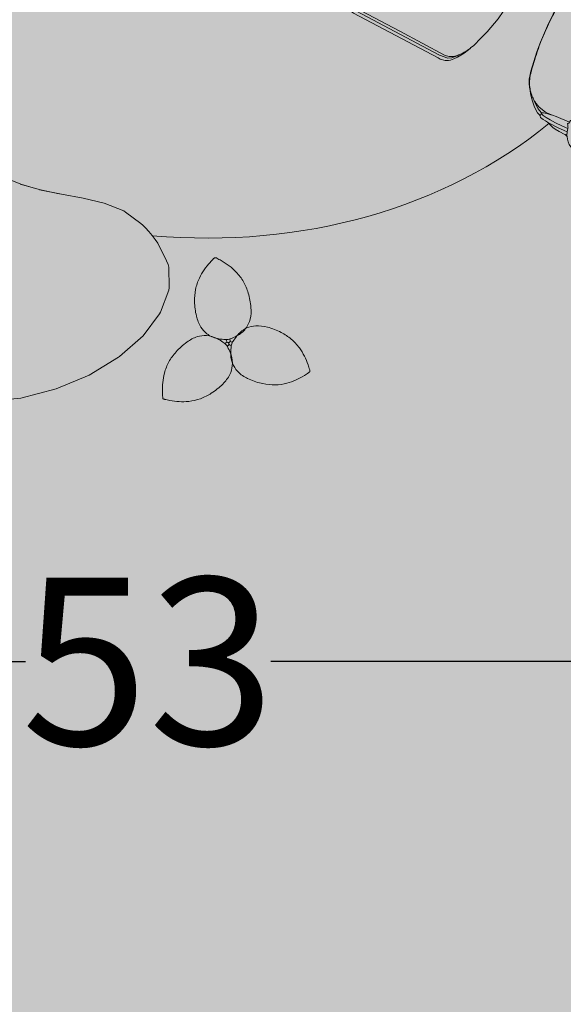
# Model space of a CAD drawing. Units: inches. Extents: x -466983 to 1020, y 324 to 318697.
# Tile 12 of 97: x 775 to 794, y 417 to 452. Entities that reach past the tile are written whole.
import ezdxf

# ---------------------------------------------------------------- set-up
doc = ezdxf.new("R2010")
doc.units = ezdxf.units.IN
doc.header["$MEASUREMENT"] = 0
for name, color, linetype, lineweight in [('A-ANNO-DIMS', 2, 'Continuous', 18), ('A-FLOR-PATT', 252, 'Continuous', 13), ('A-FURN', 8, 'Continuous', 18)]:
    doc.layers.add(name, color=color, linetype=linetype, lineweight=lineweight)
doc.layers.add('K-Hatch', color=7, linetype='Continuous')
doc.styles.get("Standard").update_dxf_attribs({"font": 'arial.ttf'})
doc.dimstyles.get("Standard").update_dxf_attribs({"dimtxt": 6, "dimasz": 4, "dimexe": 3, "dimexo": 3, "dimgap": 0.09, "dimtad": 0, "dimtih": 1, "dimtoh": 1, "dimdec": 1, "dimzin": 0, "dimdsep": 46, "dimlunit": 3, "dimtxsty": 'Standard', "dimcen": 0.09, "dimadec": 0, "dimazin": 0, "dimtfac": 1, "dimtdec": 1, "dimtofl": 0, "dimtmove": 0, "dimatfit": 3, "dimfxl": 1, "dimtolj": 1, "dimtzin": 0, "dimarcsym": 0})

# ---------------------------------------------------------------- blocks, each defined once
blk = doc.blocks.new('CBV_06')
at = {"layer": 'K-Hatch'}
h = blk.add_hatch(color=256, dxfattribs=at)
h.dxf.hatch_style = 1
h.paths.add_polyline_path([(1007.6, -162.8), (976.4, -65), (974.5, -60.9), (923.4, 38), (854.3, 132.5), (771.1, 217.3), (677.3, 287), (580.7, 342.5), (489.2, 384.4), (414.7, 413.4), (369.4, 429.9), (337.4, 440.2), (302.9, 450.6), (264.8, 460.4), (221.9, 468.5), (217.5, 469.1), (173.4, 474.9), (131.2, 477.6), (84.4, 478.5), (-21.2, 478.6), (-84.4, 478.5), (-131.2, 477.6), (-173.4, 474.9), (-217.5, 469.1), (-221.9, 468.5), (-264.8, 460.4), (-302.9, 450.6), (-337.4, 440.2), (-369.4, 429.9), (-414.7, 413.4), (-489.2, 384.4), (-580.7, 342.5), (-677.3, 287), (-771.1, 217.3), (-854.3, 132.5), (-923.4, 38), (-974.5, -60.9), (-976.4, -65), (-1007.6, -162.8), (-1016.4, -252), (-1016.2, -257.5), (-1002.7, -333.7), (-999.3, -339.8), (-963.8, -397.3), (-956.9, -403.9), (-946.2, -410.9), (-945.1, -411.6), (-892.7, -445.8), (-879.3, -451.9), (-863.7, -457.7), (-847.5, -463.3), (-832.6, -467.9), (-820.8, -470.9), (-811.5, -472.7), (-749.7, -478.5), (-742.9, -478.6), (-675.1, -467.1), (-608, -445.9), (-540.7, -420.5), (-533.5, -417.9), (-475.1, -397.7), (-450.5, -390.8), (-411.1, -379.9), (-386, -375.8), (-353.2, -370.6), (-333.2, -368.9), (-297.7, -366.2), (-239.9, -363.6), (-171.9, -362.2), (-95.5, -361.3), (-76.2, -361.4), (-13.7, -361.6), (-21.2, -361.9), (13.7, -361.6), (76.2, -361.4), (95.5, -361.3), (171.9, -362.2), (239.9, -363.6), (297.7, -366.2), (333.2, -368.9), (353.2, -370.6), (386, -375.8), (411.1, -379.9), (450.4, -390.7), (475.1, -397.7), (533.4, -417.9), (540.7, -420.5), (608, -445.9), (675.1, -467.1), (742.9, -478.6), (749.7, -478.5), (811.5, -472.7), (820.8, -470.9), (832.6, -467.9), (847.5, -463.3), (863.7, -457.7), (879.3, -451.9), (892.7, -445.8), (945.1, -411.6), (946.2, -410.9), (956.9, -403.9), (963.8, -397.3), (999.3, -339.8), (1002.7, -333.7), (1016.2, -257.5), (1016.4, -252)])
h.paths.add_polyline_path([(474.4, 70.2), (440.8, 77.6), (404.4, 87.8), (354.2, 104.4), (296.4, 124), (237, 143.3), (236.1, 143.6), (173.2, 161.3), (104.7, 175.8), (50.1, 183.8), (-6.2, 188), (-21.2, 188.7), (-32.5, 186.3), (-104.7, 175.8), (-173.2, 161.3), (-236.1, 143.6), (-237, 143.3), (-296.4, 124), (-354.2, 104.4), (-404.4, 87.8), (-440.8, 77.6), (-474.4, 70.2), (-510.8, 64.3), (-524, 62.5), (-568.6, 59.8), (-577.9, 60.2), (-570.8, 66.8), (-541.1, 87.8), (-513.8, 104.1), (-490.9, 116.3), (-470.5, 126.5), (-453.3, 134.6), (-440.4, 140.4), (-432.6, 143.7), (-427.3, 145.8), (-423.1, 147.3), (-410.5, 149.9), (-379.3, 154.4), (-338.7, 159.3), (-285, 164.8), (-220.8, 170.8), (-21.2, 189.2), (-6.2, 188), (32.5, 186.3), (50.1, 183.8), (220.8, 170.8), (285, 164.8), (338.8, 159.3), (379.3, 154.4), (410.5, 149.9), (423.1, 147.3), (427.3, 145.8), (432.6, 143.7), (440.4, 140.4), (453.3, 134.6), (470.5, 126.5), (490.9, 116.3), (513.8, 104.1), (541.1, 87.8), (570.8, 66.8), (577.9, 60.2), (568.6, 59.8), (524, 62.5), (510.8, 64.3)], flags=16)
for points in [[(472.3, -396.2), (540.7, -420.5), (608, -445.9), (675.1, -467.1), (742.9, -478.6), (749.7, -478.5), (811.5, -472.7), (820.8, -470.9), (832.6, -467.9), (847.5, -463.3), (863.7, -457.7), (879.3, -451.9), (892.7, -445.8), (946.2, -410.9), (956.9, -403.9), (963.8, -397.3), (999.3, -339.8), (1002.7, -333.7), (1016.2, -257.5), (1016.4, -252), (1007.6, -162.8), (976.4, -65), (974.5, -60.9), (923.4, 38), (854.3, 132.5), (771.1, 217.3), (677.3, 287)], [(350, -369.8), (411.1, -379.9), (450.4, -390.7)], [(408.3, -378.8), (475.1, -397.7), (533.4, -417.9)], [(892.7, -445.8), (902.5, -439.6), (946.2, -410.9), (956.9, -403.9)]]:
    blk.add_lwpolyline(points)
blk = doc.blocks.new('CBV_03')
for p, q in [((-46.9, 6), (-51.1, 6)), ((-68.8, -6.7), (-66.7, -3)), ((-58.4, -12.7), (-56.3, -9)), ((-46.9, -6), (-51.1, -6))]:
    blk.add_line(p, q)
blk.add_lwpolyline([(-68.8, 6.7), (-66.7, 3, 1), (-56.3, 9), (-58.4, 12.7)], format="xyb")
for centre, start, end in [((-61.5, -6), 330, 150), ((-51.1, 0), 90, 270)]:
    blk.add_arc(centre, 6, start, end)
for points in [[(-63.3, 9.1), (-67.2, 6.9), (-79, 3.7), (-102.2, -2.7), (-132.8, -0.8), (-164.6, 15.4), (-190.3, 45.3), (-209.9, 82.7), (-222.6, 123.3), (-223.7, 160.5), (-218.2, 193.8), (-210.3, 219.1), (-203.5, 234.1), (-201, 240.5), (-200, 242.1), (-199, 243), (-198.5, 243.3)], [(-63.3, 9.1), (-59.4, 11.4), (-50.7, 20), (-33.6, 36.9), (-19.9, 64.4), (-18.1, 100), (-31.1, 137.2), (-53.6, 172.9), (-82.5, 204.2), (-114.2, 223.8), (-145.8, 235.6), (-171.6, 241.4), (-188, 243.1), (-194.8, 244.1), (-196.7, 244), (-197.9, 243.6), (-198.5, 243.3)], [(-47.4, 0.2), (-47.5, 4.7), (-44.7, 16.6), (-39.2, 40.1), (-22.9, 66), (6.5, 86.2), (45, 94.5), (87.3, 93.9), (129.1, 85.7), (162.2, 68.9), (188.9, 48.1), (207.3, 29.2), (217.3, 16), (221.7, 10.7), (222.6, 9.1), (222.9, 7.8), (222.9, 7.2)], [(-63.3, -9.1), (-67.2, -6.9), (-79, -3.7), (-102.2, 2.7), (-132.8, 0.8), (-164.6, -15.4), (-190.3, -45.3), (-209.9, -82.7), (-222.6, -123.3), (-223.7, -160.5), (-218.2, -193.8), (-210.3, -219.1), (-203.5, -234.1), (-201, -240.5), (-200, -242.1), (-199, -243), (-198.5, -243.3)], [(-47.4, 0.2), (-47.2, -4.3), (-43.8, -16), (-37.2, -39.2), (-19.5, -64.3), (10.9, -82.9), (49.8, -89.2), (91.9, -86.5), (133.3, -76), (165.5, -57.6), (191, -35.4), (208.4, -15.6), (217.7, -1.9), (221.9, 3.6), (222.7, 5.3), (223, 6.6), (222.9, 7.2)], [(-63.3, -9.1), (-59.4, -11.4), (-50.7, -20), (-33.6, -36.9), (-19.9, -64.4), (-18.1, -100), (-31.1, -137.2), (-53.6, -172.9), (-82.5, -204.2), (-114.2, -223.8), (-145.8, -235.6), (-171.6, -241.4), (-188, -243.1), (-194.8, -244.1), (-196.7, -244), (-197.9, -243.6), (-198.5, -243.3)]]:
    blk.add_open_spline(points, degree=3, knots=[0, 0, 0, 0, 13.60379, 35.946241, 72.563034, 102.159646, 140.689545, 188.549731, 228.306921, 267.465056, 298.746796, 329.437779, 346.337038, 348.270011, 350.10195, 352.007195, 352.007195, 352.007195, 352.007195])
blk = doc.blocks.new('CBV_11')
at = {"layer": 'K-Hatch'}
h = blk.add_hatch(color=256, dxfattribs=at)
h.dxf.hatch_style = 1
h.paths.add_polyline_path([(-178.4, 698.3), (-200.4, 717.9), (-207.1, 720), (-213, 721.7), (-231.8, 722.5), (-254.2, 721.5), (-275, 717.7), (-289.3, 712.5), (-316, 699.4), (-324.9, 694.8), (-295.8, 706.5), (-286.8, 709.3), (-277.1, 712.2), (-265.3, 715), (-258.1, 715.9), (-241.3, 718.1), (-228.8, 718), (-215.5, 715.7), (-208.8, 713.2), (-205.5, 711.6), (-203.9, 710.6), (-202.4, 709.7), (-195.4, 705.2), (-194.8, 704.5), (-190.4, 699.8), (-87.3, 570), (16.1, 440.3), (19.6, 435), (22.9, 426.4), (24.1, 422.9), (25.8, 412.3), (25.1, 398.9), (24.2, 394.5), (25.6, 399.8), (28.8, 418.8), (27.5, 432), (13.6, 457)])
h.paths.add_polyline_path([(-536, 213.1), (-639.3, 342.7), (-642.9, 348.1), (-646.2, 356.7), (-647.4, 360.2), (-649.1, 370.8), (-648.4, 384.2), (-645.7, 396.4), (-637.3, 419.1), (-631.8, 430), (-626.9, 438.8), (-622.1, 446.9), (-606.5, 469.3), (-631, 439.9), (-638.6, 427.4), (-646.5, 408.6), (-652.3, 388), (-655.6, 368.8), (-654.4, 355.7), (-649, 343.1), (-640.5, 330.7), (-448.6, 89.4), (-437.6, 77.7), (-424.8, 69.2), (-413.8, 65.9), (-392.4, 64.7), (-388.1, 65), (-394.5, 65), (-407.8, 67.4), (-417, 71.1), (-420.9, 73.4), (-427.9, 77.9), (-428.5, 78.6), (-432.9, 83.2)])
for p, q in [((259, 150.4), (259, 150.4)), ((345.2, 98.6), (344, 99.3)), ((349.3, 96), (349.2, 96.1)), ((478.6, -6.2), (478.7, -6.3)), ((644.9, -391.7), (644.8, -391.9)), ((-99, -470.6), (-98.6, -470.7)), ((4, -570.8), (3.9, -570.4)), ((96.9, -581.8), (98.6, -582.5)), ((157.6, -594.8), (157.4, -595)), ((239.9, -716.7), (240.2, -716.7))]:
    blk.add_line(p, q)
for points in [[(-16.4, 313.8), (-16.1, 314.2), (2.3, 340.9), (8.8, 352.7), (9, 353), (14.8, 365.2), (18.6, 375.8), (20.5, 381.1), (22.4, 386.6), (24.2, 394.5), (25.1, 398.9), (25.8, 412.3), (24.1, 422.9), (22.9, 426.4), (19.6, 435), (16.1, 440.3), (-87.3, 570), (-190.4, 699.8), (-194.8, 704.5), (-195.4, 705.2), (-202.4, 709.7), (-203.9, 710.6), (-208.8, 713.2), (-215.5, 715.7), (-228.8, 718), (-241.3, 718.1), (-258.1, 715.9), (-265.3, 715), (-277.1, 712.2), (-286.8, 709.3), (-295.8, 706.5), (-324.9, 694.8), (-347.4, 685.7), (-397.3, 660.4), (-444.8, 630.8), (-480.8, 604.2), (-497.4, 590.5), (-534.5, 556.2), (-554.4, 535.5), (-590.2, 492.6), (-603.5, 473.5), (-606.5, 469.3), (-622.1, 446.9), (-626.9, 438.8), (-631.8, 430), (-637.3, 419.1), (-645.7, 396.4), (-648.4, 384.2), (-649.1, 370.8), (-647.4, 360.2), (-646.2, 356.7), (-642.9, 348.1), (-639.3, 342.7), (-536, 213.1), (-432.9, 83.2), (-428.5, 78.6), (-427.9, 77.9), (-420.9, 73.4), (-417, 71.1), (-407.8, 67.4), (-394.5, 65), (-388.1, 65), (-382, 64.9), (-376.6, 65.6), (-368.3, 66.6), (-367.7, 66.7), (-359.3, 67.5), (-346.5, 70.4), (-345.9, 70.6), (-336.1, 73.3), (-327.3, 76.2), (-282.4, 94.4), (-275.6, 97.1), (-225.7, 122.4), (-178.3, 151.9), (-142.2, 178.6), (-125.6, 192.2), (-88.5, 226.6), (-68.7, 247.3), (-32.9, 290.2), (-16.4, 313.8), (-16.2, 314.2)], [(9, 353), (10.3, 354.9), (16.2, 365.1), (21.5, 376.3), (26.2, 388.3), (30.1, 400.3), (33.2, 412.3), (35.5, 424.1), (35.7, 431), (33.5, 442.1), (26.2, 456.4), (21.3, 463.1), (-173.2, 707.5), (-185, 718.7), (-200.1, 726), (-205.3, 726.9), (-216.4, 727.2), (-226.1, 726.9), (-241.2, 725.8), (-253.7, 723.9), (-264.9, 721.5), (-277.2, 717.9), (-288.3, 713.3), (-311.8, 701.8), (-324.9, 694.8), (-316, 699.4), (-289.3, 712.5), (-275, 717.7), (-254.2, 721.5), (-231.8, 722.5), (-213, 721.7), (-207.1, 720), (-200.4, 717.9), (-178.4, 698.3), (13.6, 457), (27.5, 432), (28.8, 418.8), (25.6, 399.8), (24.2, 394.5)], [(-203.9, 710.6), (-205.5, 711.6), (-208.8, 713.2)], [(-346.5, 70.4), (-349.3, 69.2), (-356.8, 67), (-372.9, 63.3), (-385.5, 61.5), (-398.1, 60.5), (-410.3, 60.2), (-421.5, 60.6), (-428.5, 61.9), (-441.8, 68.9), (-453.7, 80.2), (-456.3, 83.2), (-648.2, 324.6), (-653.1, 331.3), (-657.2, 338.3), (-662.3, 353.4), (-662.3, 363.4), (-659.9, 375.1), (-656.8, 387), (-652.8, 399), (-648.1, 410.9), (-642.7, 422.1), (-636.8, 432.3), (-630.4, 441.2), (-607, 469.6), (-603.5, 473.5)], [(-606.5, 469.3), (-631, 439.9), (-638.6, 427.4), (-646.5, 408.6), (-652.3, 388), (-655.6, 368.8), (-654.4, 355.7), (-649, 343.1), (-640.5, 330.7), (-448.6, 89.4), (-437.6, 77.7), (-424.8, 69.2), (-413.8, 65.9), (-392.4, 64.7), (-388.1, 65)], [(-50.1, 67.5), (-23.5, 87.9), (-9.9, 97.6), (3.8, 107.1), (17.8, 116.4), (31.9, 125.3), (60.6, 142.4), (89.9, 158.3), (119.5, 173.3), (135, 179.9), (142.8, 182.8), (151, 184.8), (159.6, 185.9), (175.9, 186.9), (181, 186.7)], [(46.8, 133.3), (53.6, 137.3), (58.1, 140), (60.8, 141.6), (71.5, 147.3), (71.5, 147.3), (75.4, 149.5), (86.9, 155.7), (90, 157.4), (100.5, 162.5), (100.5, 162.6), (112.3, 168.5), (118.5, 171.5), (121.5, 172.9), (121.5, 172.9), (121.6, 172.9), (124.8, 174.4), (126.7, 175.2), (131.7, 177.5), (133.5, 178.2), (133.6, 178.2), (139.5, 180.3), (143.1, 181.6), (144.9, 182), (148.5, 182.9), (151.1, 183.5), (151.4, 183.6), (155.5, 184.6), (157.4, 184.8), (163.9, 185.7), (168.2, 186.2), (170.2, 186.3), (175.4, 186.4), (175.6, 186.4), (175.8, 186.4), (179.6, 186.5), (181.7, 186.3), (187.4, 185.9), (192.1, 185.5), (192.4, 185.5), (192.9, 185.4), (196.6, 184.9), (199.1, 184.5), (203, 183.5), (203.6, 183.4), (204.9, 183.1), (206.1, 182.8), (206.2, 182.8), (206.9, 182.5), (210.6, 181.4), (212.8, 180.8), (213.1, 180.7), (213.6, 180.5), (215.8, 179.8), (217.2, 179.4), (219, 178.7), (225, 176.1), (225.2, 176), (225.4, 175.9), (228.9, 174.4), (230.6, 173.5), (239.3, 168.6), (259, 150.4), (261.9, 146.4), (265.2, 141.7), (271.3, 132.8), (271.8, 133.4)], [(268, 169.8), (264.7, 172.2), (256.3, 176.5), (245.7, 180.3), (233.5, 183.5), (219.5, 185.8), (204.9, 187.1), (190.5, 187.3), (181, 186.7), (184.6, 186.6), (192.1, 185.5)], [(215.8, 179.8), (224.2, 178.5), (244.5, 172), (258.1, 164.6), (259.6, 163.4)], [(325.2, 88.8), (320.7, 95.5), (312.8, 106.8), (299.7, 124.6), (287.2, 140.3), (277.4, 151.6), (268.4, 160.4), (262.4, 164.5), (259.6, 163.6), (268, 169.8), (268.8, 170.4), (273.2, 169.7), (281.2, 162.9), (287.4, 156.5), (292.6, 150.4), (299.8, 141.9), (315.6, 121.4), (329.6, 101.6), (335.5, 92.9)], [(259.6, 163.6), (259.6, 163.4), (260.3, 157.9), (264.5, 147.6), (271, 134.8), (273.6, 130.4), (280, 119.4), (306, 80.1)], [(58.1, 140), (55.3, 138.4), (46.8, 133.3), (43.3, 131.2), (32.8, 125), (30.4, 123.5), (28, 122), (23.4, 119.1), (14, 112.9), (5.4, 107.3), (1.3, 104.5), (-2.9, 101.6), (-9.4, 97), (-9.5, 96.9), (-21, 88.8), (-24.8, 86), (-28.5, 83.3), (-36.4, 77.2), (-38.8, 75.4), (-45.1, 70.6), (-49.7, 67), (-54.2, 63.4), (-56, 61.9), (-62.5, 56.6), (-75.5, 45.6), (-77.3, 44), (-77.4, 44)], [(346.5, 95.7), (344, 99.3), (342.7, 101.1), (342.4, 101.6), (329.1, 118.9), (319.4, 130.1), (312.4, 136.8), (292.6, 150.4)], [(457.4, -155.4), (455.9, -155.5), (454.8, -155.5), (454.6, -155.5), (454.5, -155.5), (450.3, -155.2), (448.8, -154.8), (444.9, -153.5), (441.6, -151.7), (437.3, -148.8), (429.3, -140.4), (425.9, -136.3), (421.6, -130.7), (411.3, -116.8), (398.5, -99.2), (386.7, -82.7), (374.5, -65.3), (362.5, -47.8), (339.1, -12.8), (318.2, 19.8), (307.7, 36.3), (302.4, 46.9), (301.4, 48.8), (298.5, 55.5), (297.9, 58.1), (297.8, 65.2), (298.5, 67.6), (301, 75.1), (306, 80.1), (307.5, 81.6), (308.1, 82), (307.8, 84), (308.9, 85.7), (310.4, 86.8), (312.8, 87.1), (320.3, 87.9), (323, 87.9), (324.8, 88.6), (325.2, 88.8), (330.7, 91.3), (335.5, 92.9), (337.7, 93.7), (344.7, 95.5), (346.5, 95.7), (349.3, 96), (349.8, 96), (359.2, 96.9), (368.2, 95.8), (377.2, 93.8), (385.7, 90.7), (393.6, 86.2), (410.4, 73.5), (416, 68.7), (426.3, 59.8), (441.3, 45.2), (454.8, 29), (467.2, 12.1), (478.3, -5.7), (478.6, -6.2), (478.6, -6.3), (479, -7), (481, -10.8), (488.2, -24.1), (496, -43.4), (503.1, -63.4), (508.5, -83.5), (509.8, -91.8), (509.7, -100.3), (508.6, -108.6), (506.6, -116.7), (503.3, -124.2), (500, -131.2), (494.1, -139.1), (490.8, -143.5), (486.4, -147), (485.6, -147.6), (485.6, -147.6)], [(349.8, 96), (347.9, 98), (342.9, 101.1), (342.7, 101.1)], [(-217.7, -216.8), (-218.7, -214.8), (-221.6, -206), (-223.5, -195.1), (-224.4, -170.3), (-223.2, -156.5), (-220.9, -142.4), (-219, -134.5), (-218.9, -134.4), (-218.9, -134.2), (-217.3, -125.9), (-215.2, -117.7), (-212.7, -109.9), (-212.1, -108.4), (-207.7, -98.2), (-203.6, -90.8), (-196.4, -80.6), (-191.3, -74), (-180.9, -61.1), (-170.2, -48.3), (-159.1, -35.9), (-159.1, -35.8), (-148, -23.5), (-124.9, 0.7), (-113, 12.4), (-100.8, 23.9), (-88.5, 35.1), (-75.9, 46.2), (-63.1, 57), (-50.1, 67.5)], [(-214.7, -118), (-214.6, -117.8), (-212.4, -111.4), (-210.9, -107.7), (-210.4, -106.5), (-210.1, -105.7), (-209.4, -104.2), (-209, -103.5), (-206, -97.3), (-205.1, -95.8), (-204.7, -95), (-203.9, -93.8), (-203.5, -93.2), (-202.6, -91.5), (-202, -90.5), (-200.3, -88.1), (-199.3, -86.6), (-198.2, -84.9), (-198, -84.7), (-197.9, -84.5), (-192.8, -77.9), (-190.9, -75.4), (-190.5, -74.9), (-189.8, -74), (-186.5, -69.8), (-173.8, -54.2), (-170.7, -50.6), (-169.2, -48.8), (-167, -46.3), (-160.8, -39.1), (-147.5, -24.2), (-147.4, -24.1), (-147.3, -24), (-146.9, -23.6), (-146.4, -23.1), (-134, -9.8), (-127, -2.7), (-124.7, -0.3), (-124.4, -0.1), (-124.2, 0.2), (-123.2, 1.2), (-120.2, 4.2), (-106.2, 17.9), (-102.9, 20.9), (-101.4, 22.4), (-98.9, 24.6), (-91.9, 31.1), (-77.7, 43.7), (-77.6, 43.8), (-77.4, 44)], [(479, -7), (479.3, -7.2), (478.7, -6.3), (478.6, -6.3)], [(481, -10.8), (480.9, -9.4), (480, -8.1), (479.3, -7.2), (479.9, -7.7), (480, -8.1), (480, -8.6)], [(-212.1, -108.4), (-213.8, -111.2), (-223, -134.4), (-228.6, -157.2), (-231.3, -180.4), (-231, -201.3), (-228.1, -217.6), (-225.8, -223.3), (-226.1, -223.6), (-227.6, -226.1), (-224.9, -232.9), (-218.3, -243.6), (-212.6, -251.5), (-209.6, -255.8), (-197.1, -271.4), (-182.6, -288.2), (-173.4, -298.4), (-166.3, -306.1)], [(-143.8, -278.1), (-149.7, -271.9), (-151.2, -270.2), (-153.6, -267.6), (-153.7, -267.6), (-158.2, -262.7), (-179.1, -240.4), (-181.9, -237.4), (-184, -235.2), (-185.8, -233.2), (-188.4, -230.4), (-188.8, -230), (-189.2, -229.5), (-191, -227.5), (-192.6, -225.7), (-192.9, -225.2), (-193.3, -224.8), (-194.6, -223.3), (-196.5, -221), (-197, -220.3), (-197.5, -219.7), (-198.5, -218.3), (-200, -216.4), (-200.2, -216.2), (-201.3, -214.6), (-201.4, -214.5), (-203.2, -212), (-203.8, -211.2), (-204.4, -210.2), (-205.3, -208.8), (-206.1, -207.6), (-206.2, -207.4), (-206.3, -207.3), (-206.4, -207), (-206.6, -206.8), (-207.1, -206), (-207.5, -205.3), (-207.5, -205.2), (-207.6, -205.1), (-207.6, -205), (-208.1, -204.2), (-208.2, -204), (-208.3, -203.8), (-208.4, -203.7), (-208.7, -203.2), (-209.4, -202), (-209.4, -201.9), (-209.6, -201.7), (-210.3, -200.2), (-211.3, -198.2), (-211.5, -197.7), (-212.6, -194.8), (-213.7, -191.8), (-214, -190.9), (-215.6, -185.2), (-217, -180.3), (-217, -180.3), (-217, -180.3), (-217.6, -177.7), (-218.5, -172.7), (-218.9, -170.6), (-219, -169.1), (-219.2, -168.2), (-219.2, -167.9), (-219.3, -167.8), (-219.3, -166.9), (-219.6, -165), (-219.8, -163.4), (-220.2, -156.1), (-220.2, -148.7), (-219.6, -142.8), (-219.6, -142.2), (-219.6, -142), (-219.6, -141.7), (-219.5, -141.2), (-218.5, -134), (-217.9, -130.8), (-217.7, -129.5), (-217.7, -129.3), (-217.5, -128.7), (-217.5, -128.6), (-217.4, -128.4), (-217, -126.3), (-215, -118.8), (-214.9, -118.6), (-214.9, -118.5), (-214.7, -118), (-214.9, -118.5)], [(2.4, -563.5), (-3.3, -568.8), (-5, -573.7), (-2.4, -580.9), (5.2, -592.9), (5.7, -593.8), (18.8, -610.1), (45.9, -638.4), (68.4, -659.3), (96.5, -683.5), (112.7, -694.7), (124, -701.1), (147.3, -712), (166.9, -718.5), (179.8, -721.6), (199.9, -724.8), (239.8, -727.2), (268.3, -726.6), (296.4, -724), (325.3, -719.4), (352.9, -713), (380.3, -704.7), (407.4, -694.3), (433.1, -682.4), (458.3, -668.7), (482.6, -653.1), (505.7, -636), (542.7, -602.8), (575.4, -565.6), (602.5, -526.6), (625.7, -483.1), (643.9, -436.4), (652.7, -404.6), (661, -358.1), (662.3, -341.6), (662.3, -324.4), (657.8, -289.7), (648.3, -258), (641.9, -243.3), (624.1, -210.4), (611.5, -188.5), (598.9, -168.7), (586.8, -151.4), (569.2, -131.1), (563.8, -126.7), (556, -124), (545.5, -130.4)], [(155.2, -596.2), (151.6, -595.8), (147.4, -595.1), (129.4, -592.1), (123.7, -590.8), (98.6, -582.5), (97.8, -582.2), (96.9, -581.8), (74.8, -570.5), (62.9, -563.8), (52.4, -557.5), (46.9, -554.5), (42.7, -553), (37.7, -551.6), (36.8, -551.4), (31.7, -550), (21.6, -550.8), (19.3, -551.6), (10.7, -555.3), (9.9, -555.9), (4.7, -561.9), (2.4, -563.5), (3.7, -570.3), (4, -570.8), (6.8, -576.4), (8.9, -579.3), (10.2, -583.1), (17.3, -590.8), (22.7, -598.1), (36.7, -613.8), (53.2, -630.5), (71.6, -647.7), (77.1, -652.5), (77.9, -653.2), (88.3, -662.3), (97.4, -670.5), (112.3, -681.7), (138.1, -696.5), (170, -708.5), (185.7, -712.2), (201.4, -714.5), (240.2, -716.9), (281.9, -715.3), (330.8, -707.8), (377.8, -694.8), (416.2, -679.4), (459.2, -656.3), (499.4, -628.1), (521, -609.6), (541.3, -589.7), (560.1, -568.5), (577.1, -546.4), (593, -522.5), (607, -498.1), (619.2, -472.7), (629.8, -445.9), (638.3, -419.5), (645, -392), (649.6, -365.8), (651.8, -341.4), (651.9, -325.2), (649.9, -305.2), (646.3, -287), (640.9, -268.7), (640.2, -267.3), (639, -264.2), (633.6, -250.9), (617.4, -220.5), (602.1, -193.8), (587.3, -171.3), (580.6, -161.1), (567.7, -144.8), (566, -143.1), (564.1, -141.2), (554.6, -132.1), (554, -131.9), (550.5, -130.5), (549.7, -130.2), (547.6, -129.3), (545.5, -130.4), (545.4, -130.9), (538.4, -135.5), (532.9, -143.1), (531.5, -145.1), (528.5, -154.8), (529, -166.6), (529.5, -170.7), (531.1, -176.4), (534.9, -188.3), (538.2, -199.2), (543, -215.6), (547.1, -240.2), (547.6, -254.2), (546.4, -277.3), (546.2, -281.9), (545.7, -285.4), (545.4, -287.9), (545.4, -287.9), (545.3, -288.8), (545.3, -289.2), (544.3, -296.8), (542.7, -303.6), (537, -331.4), (528.9, -353.7)], [(454.6, -155.5), (454.7, -155.7), (455.1, -157.8), (455.5, -160), (455.6, -160.6), (455.6, -160.7), (456.7, -166.6), (457.5, -171.5), (458.2, -182.7), (458.6, -192.3), (458.1, -202.7), (457.9, -204.1)], [(457.4, -155.4), (457.4, -155.4), (466.4, -154.5), (471.9, -153.3), (475.6, -151.4), (481.8, -150.7), (486.4, -147), (489.4, -151.4), (501.8, -172.4), (506.9, -183.2), (511.5, -194.8), (517.3, -212.7), (523.5, -234.6), (529.9, -258.9), (536.2, -278.2), (545.2, -290)], [(461.9, -154.9), (462.2, -156.4), (462.6, -158.7), (462.7, -159.1), (462.7, -159.3), (463.8, -165.3), (464.7, -170.7), (465.4, -182.4), (465.8, -192.3), (465.4, -201.6)], [(494.1, -139.1), (498.2, -145.2), (508.4, -161.7), (516.9, -179.1), (519.8, -186.7), (527.6, -210), (534, -233), (538.1, -249.1), (543.9, -270.8), (546.4, -277.4)], [(549.7, -130.2), (547, -129.8), (545.4, -130.9)], [(-225.8, -223.3), (-218.8, -216.5), (-217.7, -216.8), (-213.1, -218.1), (-195.7, -231.2), (-175.3, -250.4), (-147.2, -280.1)], [(-159.9, -297.1), (-165.4, -291.2), (-181.5, -273.1), (-197.1, -254.2), (-203.8, -245.5), (-213.9, -230.9), (-219, -220.9), (-218.8, -216.5)], [(-212.6, -251.5), (-211.9, -253), (-204.6, -272.1), (-201.7, -277.7), (-192.5, -291.1), (-180.6, -305.8), (-175.6, -311.7), (-173.4, -314.3), (-171.3, -316.5)], [(49.6, -472.3), (49.5, -472.3), (49.1, -466.8), (46.3, -459.7), (42.7, -453.8), (36.7, -445.8), (32.2, -440.3), (21, -427.2), (-6.6, -395.6), (-20.8, -379.7), (-35.2, -364.1), (-64.1, -333.5), (-77.2, -319.8), (-92.5, -304.3), (-108.7, -288.6), (-115.6, -282.9), (-121.5, -278.5), (-131.9, -275.3), (-141.2, -276.5), (-143.8, -278.1), (-147.2, -280.1), (-148.4, -280.8), (-149.5, -281.9), (-150.1, -282.4), (-156.3, -292.9), (-159.1, -296.2), (-158.4, -292.9), (-155.5, -285.3), (-153.9, -281.9), (-151.3, -281.2), (-149.5, -281.9)], [(545.7, -285.4), (544.3, -287.1), (544, -287.5), (543.6, -287.7), (543.5, -287.7)], [(59.4, -477), (56.9, -476.1), (53.2, -474.4), (49.6, -472.8), (49.7, -473.8), (48.7, -479.4), (48, -481.2), (44.9, -489.9), (42.9, -494.4), (41, -497.8), (38.6, -502.4), (37.3, -504.2), (36.9, -504.7), (34.8, -506.8), (33.8, -507.4), (29.1, -510.5), (24.1, -512.8), (22.1, -513.7), (15.1, -516.8), (-0.5, -520.1), (-9, -519.9), (-17.2, -519.3), (-25.5, -517.5), (-33.3, -514.4), (-51.7, -504.6), (-69.5, -493.5), (-86.6, -481.2), (-95.4, -473.4), (-97.6, -471.5), (-98, -471.2), (-98.6, -470.7), (-101.4, -468.2), (-101.5, -468.1), (-102.3, -467.4), (-117.4, -452.7), (-131.1, -436.8), (-143.6, -419.9), (-154.4, -402.1), (-164.5, -383.6), (-172.5, -364.3), (-175.2, -355.6), (-176.8, -346.5), (-176.8, -337.4), (-175.1, -328.4), (-173.5, -321.4), (-172.7, -319.6), (-171.3, -316.5), (-167.5, -308.1), (-166.3, -306.1), (-163.8, -301.8), (-160.2, -297.5), (-159.9, -297.1), (-159.1, -296.2)], [(-175.6, -311.7), (-175.4, -312.6), (-174, -317.8), (-172.7, -319.6)], [(528.6, -354.6), (528.9, -353.7), (522.8, -365.4), (515.7, -377.3), (508.1, -388.2), (503.2, -394.5), (496, -403.1), (483, -417.1), (469.3, -430.9), (454.9, -444.7), (425.1, -471.8), (395, -496.8), (363.8, -520.6), (330.7, -543.5), (314.1, -554.4), (297.5, -564.7), (281, -574.1), (263.9, -582.5), (251.4, -587.6), (244.7, -589.7), (224.5, -595.3), (204.1, -597.7), (165.9, -597.3), (155.2, -596.2), (157.4, -595), (157.2, -592.9), (152.6, -587.1)], [(-101.4, -468.2), (-100.6, -469.4), (-101.3, -468.7), (-101.5, -468.1)], [(-98, -471.2), (-98.4, -471.1), (-98.9, -470.8), (-99.9, -470.3), (-100.5, -469.5), (-100.6, -469.4)], [(-97.6, -471.5), (-98.3, -471.4), (-98.9, -470.8)], [(90.8, -500.6), (86.1, -499.5), (84, -498.9), (73.3, -495), (70.3, -493.8), (55.2, -486.1), (48, -481.2)], [(99.2, -488.5), (98.9, -488.4), (88.6, -486.6), (78.5, -484.1), (68.6, -480.9), (59.4, -477), (58.2, -476.5), (57.8, -476.3), (49.6, -472.3), (49.6, -472.3), (49.6, -472.4), (49.6, -472.4), (49.6, -472.5), (49.6, -472.8)], [(147.4, -595.1), (145, -593.4), (134.3, -587.3), (109, -574.1), (88.3, -563.1), (68.7, -551.4), (57.7, -543.9), (47.9, -536.1), (44.1, -532.6), (29.2, -518.3), (24.1, -512.8), (24.1, -512.8)], [(33.8, -507.4), (37.2, -511.1), (50.6, -524.3), (64.4, -535.5), (70.8, -539.8), (90.6, -552.1), (111.2, -563.3), (124.8, -570.5), (137.6, -577.4), (152.6, -587)]]:
    blk.add_lwpolyline(points)
blk.add_lwpolyline([(536.2, -278.2, 0.060196), (503, -207.6), (501.6, -205.9), (497.9, -203.4), (490.4, -200.5), (481.7, -199.9), (471.1, -200.5), (466.7, -201.3), (465.7, -201.5), (464.5, -201.7), (461.1, -203), (457.9, -204.1), (457.5, -204.3), (457.5, -204.3), (454.5, -205.4), (446.6, -210), (444.1, -211.8), (435.9, -217.8), (427.5, -225.4), (419.3, -234.2), (396.7, -256.7), (369.9, -282.9), (360.7, -294.8), (359, -297.1), (344.2, -313.2), (323.9, -333.2), (301.6, -353), (288.9, -363.5), (265.5, -381.1), (241.1, -397.6), (216.3, -412.6), (192.3, -424.2), (160.7, -444.5), (123.2, -467.5), (113.9, -474), (106.2, -480.6), (103.9, -482.6), (100.1, -487.3), (99.2, -488.5), (96.5, -492), (94.1, -495.1), (91.8, -498.2), (91.4, -499.3), (90.8, -500.6), (90.3, -501.9), (88.1, -510.2), (87, -512.3), (85.3, -518.2), (85.1, -527), (85.8, -529.8), (88.9, -536.1, 0.065332), (140.4, -579.1)], format="xyb")
blk = doc.blocks.new('Garden Sofa')
at = {"layer": 'K-Hatch'}
h = blk.add_hatch(color=256, dxfattribs=at)
h.dxf.hatch_style = 1
h.set_gradient(color1=(0, 107, 0), color2=(0, 255, 0), name='INVSPHERICAL')
edge = h.paths.add_edge_path()
edge.add_spline(control_points=[(2455.734, 804.108), (2455.744, 804.121), (2455.819, 804.223), (2455.928, 804.471), (2455.941, 804.903), (2455.85, 805.358), (2455.677, 805.792), (2455.43, 806.116), (2455.152, 806.362), (2454.911, 806.523), (2454.749, 806.604), (2454.683, 806.641), (2454.663, 806.648), (2454.649, 806.649), (2454.642, 806.648)], knot_values=[68.031861, 68.031861, 68.031861, 68.031861, 72.563034, 102.159646, 140.689545, 188.549731, 228.306921, 267.465056, 298.746796, 329.437779, 346.337038, 348.270011, 350.10195, 352.007195, 352.007195, 352.007195, 352.007195], degree=3, periodic=0)
edge.add_spline(control_points=[(2454.642, 806.648), (2454.635, 806.646), (2454.622, 806.641), (2454.606, 806.629), (2454.554, 806.573), (2454.426, 806.446), (2454.246, 806.218), (2454.059, 805.898), (2453.924, 805.513), (2453.895, 805.046), (2453.949, 804.586), (2454.096, 804.179), (2454.302, 803.95), (2454.44, 803.863), (2454.487, 803.838)], knot_values=[58.179319, 58.179319, 58.179319, 58.179319, 60.084563, 61.916503, 63.849475, 80.748735, 111.439717, 142.721457, 181.879593, 221.636783, 269.496968, 308.026867, 337.62348, 352.007195, 352.007195, 352.007195, 352.007195], degree=3, periodic=0)
edge.add_spline(control_points=[(2454.487, 803.838), (2454.567, 803.82), (2454.644, 803.791), (2454.717, 803.754)], knot_values=[36.084782, 36.084782, 36.084782, 36.084782, 58.296883, 58.296883, 58.296883, 58.296883], degree=3, periodic=0)
edge.add_spline(control_points=[(2454.717, 803.754), (2454.717, 803.754), (2454.796, 803.736), (2454.927, 803.723), (2455.06, 803.709), (2455.109, 803.717)], knot_values=[0, 0, 0, 0, 0.019806, 22.362257, 35.966046, 35.966046, 35.966046, 35.966046], degree=3, periodic=0)
edge.add_spline(control_points=[(2455.109, 803.717), (2455.13, 803.721), (2455.15, 803.726), (2455.17, 803.733)], knot_values=[0, 0, 0, 0, 5.82512, 5.82512, 5.82512, 5.82512], degree=3, periodic=0)
edge.add_spline(control_points=[(2455.17, 803.733), (2455.197, 803.743), (2455.281, 803.78), (2455.364, 803.816), (2455.418, 803.845)], knot_values=[5.82512, 5.82512, 5.82512, 5.82512, 13.60379, 30.508356, 30.508356, 30.508356, 30.508356], degree=3, periodic=0)
edge.add_spline(control_points=[(2455.418, 803.845), (2455.431, 803.86), (2455.518, 803.966), (2455.629, 804.053), (2455.734, 804.108)], knot_values=[30.508356, 30.508356, 30.508356, 30.508356, 35.946241, 68.031861, 68.031861, 68.031861, 68.031861], degree=3, periodic=0)
h = blk.add_hatch(color=256, dxfattribs=at)
h.dxf.hatch_style = 1
h.set_gradient(color1=(0, 107, 0), color2=(0, 255, 0), name='INVSPHERICAL')
edge = h.paths.add_edge_path()
edge.add_spline(control_points=[(2458.035, 802.574), (2458.037, 802.581), (2458.039, 802.595), (2458.036, 802.615), (2458.011, 802.687), (2457.96, 802.861), (2457.846, 803.127), (2457.655, 803.445), (2457.381, 803.747), (2456.984, 803.996), (2456.554, 804.167), (2456.127, 804.233), (2455.863, 804.17), (2455.749, 804.115), (2455.734, 804.108)], knot_values=[68.031861, 68.031861, 68.031861, 68.031861, 69.937106, 71.769046, 73.702018, 90.601278, 121.29226, 152.574, 191.732136, 231.489326, 279.349511, 317.87941, 347.476023, 352.007195, 352.007195, 352.007195, 352.007195], degree=3, periodic=0)
edge.add_spline(control_points=[(2455.734, 804.108), (2455.662, 804.014), (2455.555, 803.921), (2455.436, 803.854), (2455.418, 803.845)], knot_values=[30.508356, 30.508356, 30.508356, 30.508356, 62.593976, 68.031861, 68.031861, 68.031861, 68.031861], degree=3, periodic=0)
edge.add_spline(control_points=[(2455.418, 803.845), (2455.38, 803.796), (2455.318, 803.704), (2455.254, 803.61), (2455.237, 803.563)], knot_values=[0, 0, 0, 0, 16.904566, 30.508356, 30.508356, 30.508356, 30.508356], degree=3, periodic=0)
edge.add_spline(control_points=[(2455.237, 803.563), (2455.221, 803.516), (2455.211, 803.396), (2455.201, 803.277), (2455.201, 803.208)], knot_values=[0, 0, 0, 0, 13.60379, 32.549107, 32.549107, 32.549107, 32.549107], degree=3, periodic=0)
edge.add_spline(control_points=[(2455.201, 803.208), (2455.205, 803.197), (2455.244, 803.089), (2455.264, 802.973), (2455.264, 802.87)], knot_values=[32.549107, 32.549107, 32.549107, 32.549107, 35.946241, 63.868505, 63.868505, 63.868505, 63.868505], degree=3, periodic=0)
edge.add_spline(control_points=[(2455.264, 802.87), (2455.275, 802.84), (2455.333, 802.711), (2455.508, 802.483), (2455.882, 802.266), (2456.324, 802.129), (2456.789, 802.073), (2457.192, 802.136), (2457.54, 802.262), (2457.797, 802.398), (2457.946, 802.501), (2458.01, 802.541), (2458.025, 802.556), (2458.032, 802.568), (2458.035, 802.574)], knot_values=[63.868505, 63.868505, 63.868505, 63.868505, 72.563034, 102.159646, 140.689545, 188.549731, 228.306921, 267.465056, 298.746796, 329.437779, 346.337038, 348.270011, 350.10195, 352.007195, 352.007195, 352.007195, 352.007195], degree=3, periodic=0)
h = blk.add_hatch(color=256, dxfattribs=at)
h.dxf.hatch_style = 1
h.set_gradient(color1=(0, 107, 0), color2=(0, 255, 0), name='INVSPHERICAL')
edge = h.paths.add_edge_path()
edge.add_spline(control_points=[(2454.487, 803.838), (2454.435, 803.85), (2454.274, 803.873), (2453.969, 803.832), (2453.594, 803.617), (2453.254, 803.302), (2452.973, 802.928), (2452.826, 802.547), (2452.762, 802.182), (2452.751, 801.893), (2452.766, 801.712), (2452.769, 801.636), (2452.773, 801.616), (2452.78, 801.604), (2452.785, 801.599)], knot_values=[58.296883, 58.296883, 58.296883, 58.296883, 72.563034, 102.159646, 140.689545, 188.549731, 228.306921, 267.465056, 298.746796, 329.437779, 346.337038, 348.270011, 350.10195, 352.007195, 352.007195, 352.007195, 352.007195], degree=3, periodic=0)
edge.add_spline(control_points=[(2452.785, 801.599), (2452.789, 801.593), (2452.8, 801.585), (2452.82, 801.577), (2452.894, 801.562), (2453.07, 801.519), (2453.358, 801.485), (2453.728, 801.492), (2454.127, 801.578), (2454.541, 801.797), (2454.904, 802.084), (2455.175, 802.421), (2455.257, 802.697), (2455.264, 802.838), (2455.264, 802.87)], knot_values=[63.868505, 63.868505, 63.868505, 63.868505, 65.77375, 67.60569, 69.538662, 86.437922, 117.128904, 148.410644, 187.56878, 227.32597, 275.186155, 313.716054, 343.312667, 352.007195, 352.007195, 352.007195, 352.007195], degree=3, periodic=0)
edge.add_spline(control_points=[(2455.264, 802.87), (2455.227, 802.966), (2455.204, 803.081), (2455.201, 803.196), (2455.201, 803.208)], knot_values=[32.549107, 32.549107, 32.549107, 32.549107, 60.471371, 63.868505, 63.868505, 63.868505, 63.868505], degree=3, periodic=0)
edge.add_spline(control_points=[(2455.201, 803.208), (2455.177, 803.273), (2455.134, 803.36), (2455.092, 803.448), (2455.078, 803.472)], knot_values=[6.047046, 6.047046, 6.047046, 6.047046, 24.992363, 32.549107, 32.549107, 32.549107, 32.549107], degree=3, periodic=0)
edge.add_spline(control_points=[(2455.078, 803.472), (2455.067, 803.491), (2455.054, 803.51), (2455.04, 803.527)], knot_values=[0, 0, 0, 0, 6.047046, 6.047046, 6.047046, 6.047046], degree=3, periodic=0)
edge.add_spline(control_points=[(2455.04, 803.527), (2455.026, 803.543), (2455.009, 803.558), (2454.992, 803.572)], knot_values=[0, 0, 0, 0, 6.047046, 6.047046, 6.047046, 6.047046], degree=3, periodic=0)
edge.add_spline(control_points=[(2454.992, 803.572), (2454.971, 803.59), (2454.88, 803.653), (2454.79, 803.716), (2454.717, 803.754), (2454.717, 803.754)], knot_values=[6.047046, 6.047046, 6.047046, 6.047046, 13.60379, 35.946241, 36.084782, 36.084782, 36.084782, 36.084782], degree=3, periodic=0)
edge.add_spline(control_points=[(2454.717, 803.754), (2454.637, 803.772), (2454.56, 803.8), (2454.487, 803.838)], knot_values=[35.966046, 35.966046, 35.966046, 35.966046, 58.179319, 58.179319, 58.179319, 58.179319], degree=3, periodic=0)
at = {"extrusion": (0, 0, -1)}
blk.add_ellipse((2450.434, 828.917), major_axis=(18.681, -14.923), ratio=0.833526, start_param=6.462993, end_param=7.179107, dxfattribs=at)
at = {"xscale": -0.0109740885734132, "yscale": 0.0109740885734132, "zscale": 0.0109740885734132}
for name, p, rotation in [('CBV_11', (2467.574, 814.959), 100.5267845499335), ('CBV_06', (2441.681, 808.037), 148.8828363109627), ('CBV_03', (2455.012, 804.228), 280.5267845499334)]:
    blk.add_blockref(name, p, dxfattribs=dict(at, rotation=rotation))
blk = doc.blocks.new('*D93')
at = {"layer": 'A-ANNO-DIMS', "color": 0, "lineweight": -2, "transparency": 16777216}
for p, q in [((808.966, 500.777), (818.266, 500.777)), ((815.266, 496.777), (815.266, 472.969)), ((815.266, 442.777), (815.266, 466.584)), ((808.966, 438.777), (818.266, 438.777))]:
    blk.add_line(p, q, dxfattribs=at)
at = {"layer": 'A-ANNO-DIMS', "color": 0, "transparency": 16777216}
for points in [[(814.599, 496.777), (815.933, 496.777), (815.266, 500.777)], [(814.599, 442.777), (815.933, 442.777), (815.266, 438.777)]]:
    blk.add_solid(points, dxfattribs=at)
at = {"layer": 'Defpoints', "color": 0, "transparency": 16777216}
for p in [(805.966, 500.777), (815.266, 500.777), (805.966, 438.777)]:
    blk.add_point(p, dxfattribs=at)
at = {"layer": 'A-ANNO-DIMS', "color": 0, "transparency": 16777216, "insert": (815.266, 469.777), "char_height": 6, "attachment_point": 5}
blk.add_mtext('\\A1;GARDEN SEAT 62', dxfattribs=at)
blk = doc.blocks.new('*D94')
at = {"layer": 'A-ANNO-DIMS', "color": 0, "lineweight": -2, "transparency": 16777216}
for p, q in [((753.135, 435.777), (753.135, 426.477)), ((805.966, 435.777), (805.966, 426.477)), ((757.135, 429.477), (775.163, 429.477)), ((801.966, 429.477), (783.938, 429.477))]:
    blk.add_line(p, q, dxfattribs=at)
at = {"layer": 'A-ANNO-DIMS', "color": 0, "transparency": 16777216}
for points in [[(757.135, 430.143), (757.135, 428.81), (753.135, 429.477)], [(801.966, 430.143), (801.966, 428.81), (805.966, 429.477)]]:
    blk.add_solid(points, dxfattribs=at)
at = {"layer": 'Defpoints', "color": 0, "transparency": 16777216}
for p in [(753.135, 438.777), (805.966, 438.777), (805.966, 429.477)]:
    blk.add_point(p, dxfattribs=at)
at = {"layer": 'A-ANNO-DIMS', "color": 0, "transparency": 16777216, "insert": (779.551, 429.477), "char_height": 6, "attachment_point": 5}
blk.add_mtext('\\A1;53', dxfattribs=at)
blk = doc.blocks.new('*D97')
at = {"layer": 'A-ANNO-DIMS', "color": 0, "lineweight": -2, "transparency": 16777216}
for p, q in [((823.929, 568.441), (802.329, 568.441)), ((805.329, 564.441), (805.329, 499.545)), ((805.329, 428.441), (805.329, 493.337)), ((823.929, 424.441), (802.329, 424.441))]:
    blk.add_line(p, q, dxfattribs=at)
at = {"layer": 'A-ANNO-DIMS', "color": 0, "transparency": 16777216}
for points in [[(804.662, 564.441), (805.996, 564.441), (805.329, 568.441)], [(804.662, 428.441), (805.996, 428.441), (805.329, 424.441)]]:
    blk.add_solid(points, dxfattribs=at)
at = {"layer": 'Defpoints', "color": 0, "transparency": 16777216}
for p in [(826.929, 568.441), (805.329, 424.441), (826.929, 424.441)]:
    blk.add_point(p, dxfattribs=at)
at = {"layer": 'A-ANNO-DIMS', "color": 0, "transparency": 16777216, "insert": (805.329, 496.441), "char_height": 6, "attachment_point": 5}
blk.add_mtext('\\A1;BIKE 144', dxfattribs=at)

msp = doc.modelspace()

# ---------------------------------------------------------------- hatches: boundary and pattern name
at = {"layer": 'A-FLOR-PATT', "transparency": 33554661}
h = msp.add_hatch(color=256, dxfattribs=at)
h.dxf.hatch_style = 1
h.set_gradient(color1=(19, 155, 72), color2=(0, 107, 0), name='CYLINDER')
h.paths.add_polyline_path([(813.806, 503.938), (730.806, 503.938), (730.806, 424.938), (612.806, 424.938), (612.806, 415.938), (442.806, 415.938), (442.806, 368.938), (813.806, 368.938)])
h.paths.add_polyline_path([(771.796, 407.07), (783.796, 407.07), (783.796, 371.07), (771.796, 371.07)], flags=16)
h.paths.add_polyline_path([(755.796, 407.07), (755.796, 371.07), (743.796, 371.07), (743.796, 407.07)], flags=16)
h.paths.add_polyline_path([(769.796, 404.07), (769.796, 374.07), (757.796, 374.07), (757.796, 404.07)], flags=16)
h.paths.add_polyline_path([(785.796, 404.07), (797.796, 404.07), (797.796, 374.07), (785.796, 374.07)], flags=16)
h.paths.add_polyline_path([(741.796, 404.07), (741.796, 374.07), (729.796, 374.07), (729.796, 404.07)], flags=16)
h.paths.add_polyline_path([(799.796, 407.07), (811.796, 407.07), (811.796, 371.07), (799.796, 371.07)], flags=16)
h.paths.add_polyline_path([(727.796, 407.07), (727.796, 371.07), (715.796, 371.07), (715.796, 407.07)], flags=16)
h.paths.add_polyline_path([(713.796, 404.07), (713.796, 374.07), (701.796, 374.07), (701.796, 404.07)], flags=16)
h.paths.add_polyline_path([(699.796, 407.07), (699.796, 371.07), (687.796, 371.07), (687.796, 407.07)], flags=16)
h.paths.add_polyline_path([(685.796, 404.07), (685.796, 374.07), (673.796, 374.07), (673.796, 404.07)], flags=16)
h.paths.add_polyline_path([(671.796, 407.07), (671.796, 371.07), (659.796, 371.07), (659.796, 407.07)], flags=16)
h.paths.add_polyline_path([(657.796, 404.07), (657.796, 374.07), (645.796, 374.07), (645.796, 404.07)], flags=16)
h.paths.add_polyline_path([(643.796, 407.07), (643.796, 371.07), (631.796, 371.07), (631.796, 407.07)], flags=16)
h.paths.add_polyline_path([(629.796, 404.07), (629.796, 374.07), (617.796, 374.07), (617.796, 404.07)], flags=16)
h.paths.add_polyline_path([(615.796, 407.07), (615.796, 371.07), (603.796, 371.07), (603.796, 407.07)], flags=16)
h.paths.add_polyline_path([(601.796, 404.07), (601.796, 374.07), (589.796, 374.07), (589.796, 404.07)], flags=16)
at = {"layer": 'A-FLOR-PATT'}
h = msp.add_hatch(dxfattribs=at)
h.set_pattern_fill('GRASS', color=256, scale=6)
h.set_pattern_definition([(90, (-1212.4137, -290.035), (-4.242641, 4.242641), [1.125, -7.360281]), (45, (-1212.4137, -290.035), (-4.24264, 4.24264), [1.125, -4.875]), (135, (-1212.4137, -290.035), (-4.24264, -4.24264), [1.125, -4.875])])
h.paths.add_polyline_path([(813.806, 503.938), (730.806, 503.938), (730.806, 424.938), (612.806, 424.938), (612.806, 415.938), (442.806, 415.938), (442.806, 368.938), (813.806, 368.938)])
h.paths.add_polyline_path([(589.796, 404.07), (601.796, 404.07), (601.796, 374.07), (589.796, 374.07)], flags=16)
h.paths.add_polyline_path([(603.796, 407.07), (615.796, 407.07), (615.796, 371.07), (603.796, 371.07)], flags=16)
h.paths.add_polyline_path([(617.796, 404.07), (629.796, 404.07), (629.796, 374.07), (617.796, 374.07)], flags=16)
h.paths.add_polyline_path([(631.796, 407.07), (643.796, 407.07), (643.796, 371.07), (631.796, 371.07)], flags=16)
h.paths.add_polyline_path([(645.796, 404.07), (657.796, 404.07), (657.796, 374.07), (645.796, 374.07)], flags=16)
h.paths.add_polyline_path([(659.796, 407.07), (671.796, 407.07), (671.796, 371.07), (659.796, 371.07)], flags=16)
h.paths.add_polyline_path([(673.796, 404.07), (685.796, 404.07), (685.796, 374.07), (673.796, 374.07)], flags=16)
h.paths.add_polyline_path([(687.796, 407.07), (699.796, 407.07), (699.796, 371.07), (687.796, 371.07)], flags=16)
h.paths.add_polyline_path([(701.796, 404.07), (713.796, 404.07), (713.796, 374.07), (701.796, 374.07)], flags=16)
h.paths.add_polyline_path([(715.796, 407.07), (727.796, 407.07), (727.796, 371.07), (715.796, 371.07)], flags=16)
h.paths.add_polyline_path([(729.796, 404.07), (741.796, 404.07), (741.796, 374.07), (729.796, 374.07)], flags=16)
h.paths.add_polyline_path([(743.796, 407.07), (755.796, 407.07), (755.796, 371.07), (743.796, 371.07)], flags=16)
h.paths.add_polyline_path([(757.796, 404.07), (769.796, 404.07), (769.796, 374.07), (757.796, 374.07)], flags=16)
h.paths.add_polyline_path([(771.796, 407.07), (783.796, 407.07), (783.796, 371.07), (771.796, 371.07)], flags=16)
h.paths.add_polyline_path([(785.796, 404.07), (797.796, 404.07), (797.796, 374.07), (785.796, 374.07)], flags=16)
h.paths.add_polyline_path([(799.796, 407.07), (811.796, 407.07), (811.796, 371.07), (799.796, 371.07)], flags=16)

# ---------------------------------------------------------------- block references
at = {"layer": 'A-FURN'}
msp.add_blockref('Garden Sofa', (-1672.7, -362.711), dxfattribs=at)

# ---------------------------------------------------------------- dimensions: what is measured, and where the dimension line sits
at = {"layer": 'A-ANNO-DIMS'}
for base, p1, p2, angle, text, picture, middle in [((805.329, 424.441), (826.929, 568.441), (826.929, 424.441), 270, 'BIKE <>', '*D97', (805.329, 496.441)), ((815.266, 500.777), (805.966, 438.777), (805.966, 500.777), 90, 'GARDEN SEAT <>', '*D93', (815.266, 469.777))]:
    dim = msp.add_linear_dim(base=base, p1=p1, p2=p2, angle=angle, text=text, dimstyle='Standard', override={"dimdec": 0, "dimlfac": 1, "dimrnd": 0, "dimzin": 0, "dimdsep": 46, "dimlunit": 2}, dxfattribs=at)
    dim.commit()
    dim.dimension.update_dxf_attribs({"geometry": picture, "text_midpoint": middle})
dim = msp.add_linear_dim(base=(805.966, 429.477), p1=(753.135, 438.777), p2=(805.966, 438.777), dimstyle='Standard', override={"dimdec": 0, "dimlfac": 1, "dimrnd": 0, "dimzin": 0, "dimdsep": 46, "dimlunit": 2}, dxfattribs=at)
dim.commit()
dim.dimension.update_dxf_attribs({"geometry": '*D94', "text_midpoint": (779.551, 429.477)})

doc.saveas('drawing.dxf')
